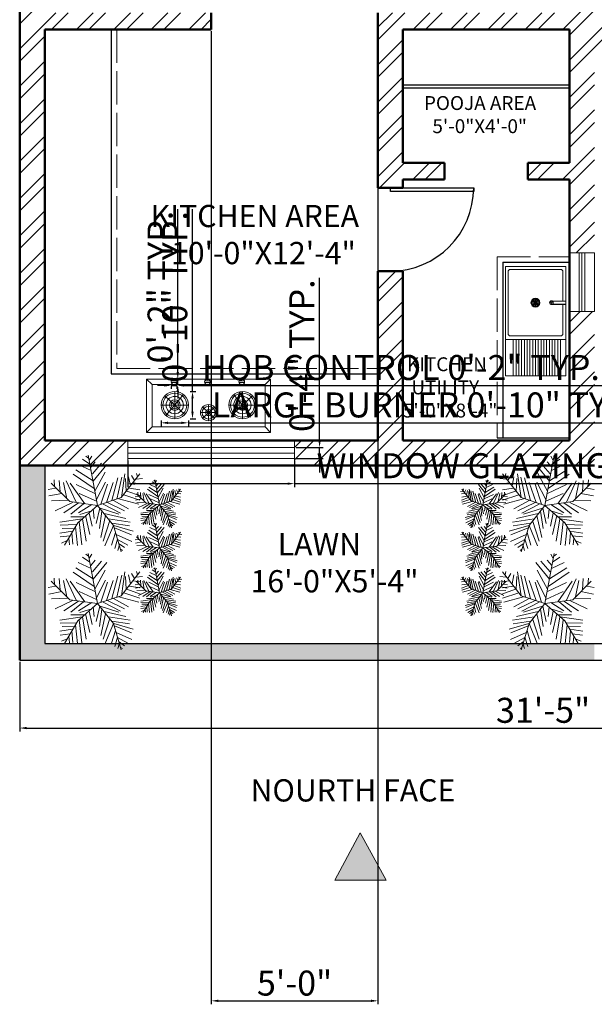
# Model space of a CAD drawing. Units: inches. Extents: x 764 to 1199, y 2696 to 3678.
# Tile 1 of 3: x 777 to 984, y 2696 to 3051. Entities that reach past the tile are written whole.
import ezdxf

# ---------------------------------------------------------------- set-up
doc = ezdxf.new("R2010")
doc.units = ezdxf.units.IN
doc.linetypes.add('ACAD_ISO02W100', pattern=[15, 12, -3])
for name, color, linetype, lineweight in [('A-ANNO-DIMS', 2, 'Continuous', 18), ('A-ANNO-SYMB', 7, 'Continuous', 18), ('A-ANNO-TEXT', 7, 'Continuous', 18), ('A-AREA-IDEN', 7, 'Continuous', 18), ('A-DOOR', 4, 'Continuous', 25), ('A-EQPM', 9, 'Continuous', 18), ('A-FIXT-PATT', 8, 'Continuous', 13), ('A-FLOR-FIXT', 8, 'Continuous', 20), ('A-GLAZ', 244, 'Continuous', 20), ('A-MILL', 8, 'Continuous', 25), ('A-MILL-HIDN', 8, 'ACAD_ISO02W100', 13), ('A-WALL', 7, 'Continuous', 50), ('A-WALL-PATT', 252, 'Continuous', 13), ('L-HRDS', 7, 'Continuous', 30), ('L-PLNT', 3, 'Continuous', 13)]:
    doc.layers.add(name, color=color, linetype=linetype, lineweight=lineweight)
doc.styles.get("Standard").update_dxf_attribs({"font": 'arial.ttf'})
doc.dimstyles.new('ISO-25', dxfattribs={"dimtxt": 9, "dimasz": 2.5, "dimexe": 1.25, "dimexo": 0.625, "dimtad": 1, "dimlunit": 3, "dimtxsty": 'Standard', "dimcen": 2.5, "dimadec": 0, "dimazin": 0, "dimtfac": 1, "dimtmove": 0, "dimatfit": 3, "dimfxl": 1, "dimarcsym": 0})

# ---------------------------------------------------------------- blocks, each defined once
blk = doc.blocks.new('*U5')
for p, q in [((-40, -1.47e-14), (-40, 5.999999999999984)), ((0, 0), (0, 5.999999999999999))]:
    blk.add_line(p, q)
blk.add_lwpolyline([(0, 0), (7.1e-15, -40), (-1.749999999999992, -40), (-1.75, -1e-16)], close=True)
blk.add_arc((0, 0), 40, 180, 270)
blk = doc.blocks.new('*U13')
for p, q in [((-10.18600000000015, 53.63999999999987), (-13.08399999999983, 55.96199999999976)), ((0, 0), (-10.5, 57)), ((-9.098999999999705, 51.7819999999997), (-6.563000000000101, 55.96199999999976)), ((-7.28800000000001, 39.70699999999965), (-21.77800000000025, 46.67299999999977)), ((-8.736999999999625, 47.13799999999969), (-17.06899999999996, 52.71100000000001)), ((-7.65000000000009, 43.42299999999977), (-2.577999999999974, 49.45999999999981)), ((-5.838999999999941, 35.99199999999973), (4.666999999999916, 48.06699999999977)), ((-5.114000000000032, 27.63199999999983), (10.46300000000019, 46.67299999999977)), ((-3.665000000000418, 19.27299999999968), (-27.57400000000007, 35.52699999999982)), ((-5.114000000000032, 28.09699999999975), (-24.67599999999993, 40.63599999999996)), ((-2.940999999999803, 16.48599999999987), (8.652000000000044, 37.84999999999991)), ((27, 9), (48, 36)), ((27.12699999999995, 9.05600000000004), (31.11200000000008, 35.99199999999973)), ((38.71900000000005, 34.13399999999979), (41.97899999999981, 28.56099999999992)), ((44.15300000000025, 36.45599999999991), (45.23900000000003, 32.74099999999999)), ((-31.5, 4.5), (-52.5, 25.5)), ((-48.58500000000003, 21.13099999999986), (-49.30899999999974, 29.02600000000007)), ((-43.51299999999992, 28.56099999999992), (-42.42699999999968, 15.55799999999976)), ((-38.44199999999955, 26.23899999999981), (-34.81899999999996, 7.662999999999783)), ((-35.54399999999987, 28.09699999999975), (-24.31399999999985, 3.946999999999661)), ((-14.5329999999999, 2.089999999999918), (-30.83399999999983, 25.30999999999995)), ((-24.31399999999985, 23.91699999999969), (-2.940999999999803, 13.69999999999982)), ((-1.128999999999905, 6.733999999999923), (9.014000000000124, 26.70399999999995)), ((3.942000000000007, 1.625), (11.1869999999999, 24.38099999999986)), ((10.10100000000011, 3.482999999999719), (17.70800000000008, 26.23899999999981)), ((16.25900000000001, 5.804999999999836), (23.14199999999983, 31.34799999999973)), ((22.05499999999984, 7.197999999999865), (27.48900000000003, 32.27699999999982)), ((31.83600000000024, 30.88299999999981), (32.56100000000015, 16.48599999999987)), ((35.09600000000001, 32.74099999999999), (37.26999999999998, 22.52399999999989)), ((40.52999999999975, 25.77499999999986), (48.86200000000008, 24.846)), ((43.79100000000017, 29.95399999999995), (51.03600000000006, 30.88299999999981)), ((-47.49800000000004, 19.73699999999962), (-55.83000000000038, 18.34399999999982)), ((-40.61500000000023, 13.69999999999982), (-55.10500000000002, 10.91299999999978)), ((-20.69099999999981, 13.69999999999982), (-1.128999999999905, 4.875999999999976)), ((29.66199999999981, 12.30699999999979), (48.13699999999972, 6.268999999999778)), ((33.28499999999986, 16.48599999999987), (48.86200000000008, 10.91299999999978)), ((36.18300000000045, 19.73699999999962), (48.13699999999972, 17.87999999999988)), ((-33.37000000000035, 6.268999999999778), (-52.20699999999988, 5.339999999999918)), ((-28.29899999999998, 3.482999999999719), (-47.86000000000012, -5.805000000000063)), ((-21.41600000000017, 3.017999999999801), (-38.07899999999973, -8.128000000000384)), ((0, 0), (-31.5, 4.5)), ((-15.98199999999951, 2.089999999999918), (-30.11000000000013, -9.521000000000186)), ((0, 0), (-22.5, -19.5)), ((-6.563000000000101, 1.161000000000058), (-21.41600000000017, -8.128000000000384)), ((0, 0), (27, 9)), ((0, 0), (18, -22.5)), ((6.478000000000065, 1.625), (26.03999999999996, -8.592000000000326)), ((11.1869999999999, 3.482999999999719), (30.74900000000025, -5.805000000000063)), ((18.06999999999971, 5.804999999999836), (35.09600000000001, -3.483000000000174)), ((24.22899999999982, 7.662999999999783), (46.6880000000001, 1.625)), ((-6.563000000000101, -5.805000000000063), (-19.96699999999964, -9.985000000000127)), ((-9.460999999999785, -8.592000000000326), (-6.201000000000021, -23.4530000000002)), ((-4.751999999999952, -3.483000000000174), (-3.665000000000418, -14.62900000000013)), ((2.493000000000392, -3.019000000000005), (-1.490999999999985, -20.20200000000023)), ((1.769000000000232, -2.555000000000063), (24.22899999999982, -9.521000000000186)), ((5.028999999999996, -6.270000000000209), (2.131000000000312, -25.77500000000009)), ((7.564999999999599, -9.056000000000267), (32.19800000000032, -14.62900000000013)), ((-17.43100000000004, -15.09400000000005), (-42.78899999999976, -18.80899999999997)), ((-24.31399999999985, -21.59600000000023), (-42.42699999999968, -22.06000000000017)), ((-22.5, -19.5), (-37.5, -45)), ((-15.2569999999996, -12.77200000000016), (-30.11000000000013, -12.77200000000016)), ((-20.69099999999981, -18.34500000000003), (-17.79300000000012, -44.35200000000032)), ((-17.06899999999996, -15.09400000000005), (-12.721, -40.17200000000025)), ((-13.44599999999991, -11.37800000000038), (-8.736999999999625, -32.74100000000021)), ((9.014000000000124, -11.37800000000038), (3.579999999999927, -35.99200000000019)), ((14.08499999999958, -16.95100000000025), (6.478000000000065, -40.17200000000025)), ((12.27399999999988, -15.09400000000005), (36.9069999999997, -18.80899999999997)), ((16.25900000000001, -19.73800000000028), (36.18300000000045, -22.98900000000003)), ((-28.29899999999998, -29.02600000000007), (-42.78899999999976, -31.34800000000018)), ((-26.8489999999997, -26.24000000000001), (-40.25300000000015, -25.77500000000009)), ((-29.02300000000014, -30.88400000000002), (-27.93600000000015, -43.88700000000016)), ((-25.03800000000001, -23.91800000000035), (-22.86500000000024, -45.28100000000017)), ((18.06999999999971, -22.52400000000012), (8.289000000000215, -45.74500000000012)), ((20.24400000000014, -30.4190000000001), (15.89699999999993, -44.81600000000026)), ((18, -22.5), (27, -52.5)), ((18.43300000000045, -22.52400000000012), (40.52999999999975, -29.02600000000007)), ((19.1569999999997, -25.31100000000015), (38.71900000000005, -33.20600000000013)), ((21.33100000000013, -32.74100000000021), (39.08100000000013, -40.63600000000019)), ((-30.83399999999983, -34.13499999999999), (-42.42699999999968, -35.52800000000025)), ((-34.45699999999988, -39.70800000000031), (-40.97800000000006, -42.49400000000014)), ((-32.64600000000019, -36.92100000000005), (-31.92099999999982, -44.35200000000032)), ((22.77999999999975, -37.85000000000014), (19.51900000000023, -48.53200000000015)), ((22.77999999999975, -38.31400000000008), (34.37199999999985, -44.81600000000026)), ((24.59100000000035, -43.42300000000022), (30.74900000000025, -47.60300000000029)), ((24.59100000000035, -45.74500000000012), (23.14199999999983, -50.85400000000004)), ((26.76400000000012, -49.92500000000018), (28.21300000000019, -50.85400000000004))]:
    blk.add_line(p, q)
blk = doc.blocks.new('*D14')
at = {"layer": 'A-ANNO-DIMS', "color": 0, "lineweight": -2, "transparency": 16777216}
for p, q in [((777.2372615392014, 2819.625478579777), (777.2372615392014, 2794.515568669596)), ((1154.237261539201, 2819.625478579777), (1154.237261539201, 2794.515568669596)), ((779.7372615392014, 2795.765568669596), (1151.737261539201, 2795.765568669596))]:
    blk.add_line(p, q, dxfattribs=at)
at = {"layer": 'A-ANNO-DIMS', "color": 0, "transparency": 16777216}
for points in [[(779.7372615392014, 2796.182235336263), (779.7372615392014, 2795.34890200293), (777.2372615392014, 2795.765568669596)], [(1151.737261539201, 2796.182235336263), (1151.737261539201, 2795.34890200293), (1154.237261539201, 2795.765568669596)]]:
    blk.add_solid(points, dxfattribs=at)
at = {"layer": 'Defpoints', "color": 0, "transparency": 16777216}
for p in [(777.2372615392014, 2820.250478579778), (1154.237261539201, 2820.250478579778), (1154.237261539201, 2795.765568669596)]:
    blk.add_point(p, dxfattribs=at)
at = {"layer": 'A-ANNO-DIMS', "color": 0, "transparency": 16777216, "insert": (965.7372615392015, 2800.988795136172), "char_height": 9, "attachment_point": 5}
blk.add_mtext('31\'-5"', dxfattribs=at)
blk = doc.blocks.new('WIN-GLAZING-60IN')
for p, q in [((0.0002615392013468, 4.000478579777791), (60.00026153920135, 4.000478579777791)), ((0.0002615392013468, 2.000478579777791), (60.00026153920135, 2.000478579777791)), ((0.0002615392013468, 0.0004785797777913), (60.00026153920135, 0.0004785797777913))]:
    blk.add_line(p, q)
blk = doc.blocks.new('VENT-GLAZING-21IN')
for p, q in [((0.0002615392015741, 0.0004785797773366), (0.0002615392015741, 21.00047857977734)), ((1.000261539201574, 0.0004785797773366), (1.000261539201574, 21.00047857977734)), ((2.000261539201574, 0.0004785797773366), (2.000261539201574, 21.00047857977734))]:
    blk.add_line(p, q)
blk = doc.blocks.new('COOKTOP-BURNER-LARGE')
for p, q in [((8.519274616664575, 1.570641359189266), (1.313840023247735, 8.261224759886773)), ((1.758228681000105, 1.148240305507442), (8.074885958912205, 8.683625813568597)), ((4.916557319956154, 9.832288262371094), (4.916557319956154, -0.0004221432950544)), ((0.0002021171230808, 4.915933059538019), (9.83291252278923, 4.915933059538019))]:
    blk.add_line(p, q)
for radius in [4.916355202833074, 4.316355202833074, 3.116355202833074, 1.916355202833074, 1.316355202833074]:
    blk.add_circle((4.916557319956154, 4.915933059538019), radius)
blk = doc.blocks.new('COOKTOP-CONTROL')
for p, q in [((0.0453271065459831, 1.317444336811149), (1.989388325886238, 1.317444336811604)), ((0.0453271065460967, 0.7174443368112406), (1.989388325886238, 0.7174443368112406))]:
    blk.add_line(p, q)
blk.add_circle((1.01735771621611, 1.017444336811422), 1.017272582022997)
for start, end in [(45.96822923670138, 134.0317707633033), (225.9682292368025, 314.0317707631974)]:
    blk.add_arc((1.01735771621611, 1.017444336811422), 0.4172725820229971, start, end)
blk = doc.blocks.new('*D24')
at = {"layer": 'A-ANNO-DIMS', "color": 0, "lineweight": -2, "transparency": 16777216}
for p, q in [((816.2372615392019, 2892.125478579778), (816.2372615392019, 2882.500478579778)), ((876.237261539202, 2892.125478579778), (876.237261539202, 2882.500478579778)), ((818.7372615392019, 2883.750478579778), (873.737261539202, 2883.750478579778)), ((876.237261539202, 2883.750478579778), (1052.558885004413, 2883.750478579778))]:
    blk.add_line(p, q, dxfattribs=at)
at = {"layer": 'A-ANNO-DIMS', "color": 0, "transparency": 16777216}
for points in [[(818.7372615392019, 2884.167145246444), (818.7372615392019, 2883.333811913111), (816.2372615392019, 2883.750478579778)], [(873.737261539202, 2884.167145246444), (873.737261539202, 2883.333811913111), (876.237261539202, 2883.750478579778)]]:
    blk.add_solid(points, dxfattribs=at)
at = {"layer": 'Defpoints', "color": 0, "transparency": 16777216}
for p in [(816.2372615392019, 2892.750478579778), (876.237261539202, 2892.750478579778), (876.237261539202, 2883.750478579778)]:
    blk.add_point(p, dxfattribs=at)
at = {"layer": 'A-ANNO-DIMS', "color": 0, "transparency": 16777216, "insert": (965.6480732718076, 2889.032027010883), "char_height": 9, "attachment_point": 5}
blk.add_mtext('WINDOW GLAZING 5\'-0" TYP.', dxfattribs=at)
blk = doc.blocks.new('*D25')
at = {"layer": 'A-ANNO-DIMS', "color": 0, "lineweight": -2, "transparency": 16777216}
for p, q in [((885.2372615392029, 2899.250478579779), (885.2372615392029, 2957.859960162317)), ((876.8622615392024, 2896.750478579779), (886.4872615392028, 2896.750478579779)), ((885.2372615392029, 2892.750478579779), (885.2372615392029, 2896.750478579779)), ((876.8622615392024, 2892.750478579779), (886.4872615392028, 2892.750478579779)), ((885.2372615392029, 2890.250478579779), (885.2372615392029, 2887.750478579779))]:
    blk.add_line(p, q, dxfattribs=at)
at = {"layer": 'A-ANNO-DIMS', "color": 0, "transparency": 16777216}
for points in [[(884.8205948725363, 2899.250478579779), (885.6539282058696, 2899.250478579779), (885.2372615392029, 2896.750478579779)], [(884.8205948725363, 2890.250478579779), (885.6539282058696, 2890.250478579779), (885.2372615392029, 2892.750478579779)]]:
    blk.add_solid(points, dxfattribs=at)
at = {"layer": 'Defpoints', "color": 0, "transparency": 16777216}
for p in [(876.2372615392024, 2896.750478579779), (885.2372615392029, 2896.750478579779), (876.2372615392024, 2892.750478579779)]:
    blk.add_point(p, dxfattribs=at)
at = {"layer": 'A-ANNO-DIMS', "color": 0, "transparency": 16777216, "insert": (880.0171046497084, 2929.805219371047), "char_height": 9, "attachment_point": 5, "rotation": 90}
blk.add_mtext('0\'-4" TYP.', dxfattribs=at)
blk = doc.blocks.new('*D28')
at = {"layer": 'A-ANNO-DIMS', "color": 0, "lineweight": -2, "transparency": 16777216}
for p, q in [((829.3360851341931, 2919.092989980183), (826.8360851341931, 2919.092989980183)), ((831.8360851341932, 2919.092989980183), (833.8706302982391, 2919.092989980183)), ((831.8360851341932, 2918.77317175479), (831.8360851341932, 2917.842989980183)), ((833.8706302982391, 2918.77317175479), (833.8706302982391, 2917.842989980183)), ((836.3706302982391, 2919.092989980183), (990.1983929176115, 2919.092989980183))]:
    blk.add_line(p, q, dxfattribs=at)
at = {"layer": 'A-ANNO-DIMS', "color": 0, "transparency": 16777216}
for points in [[(829.3360851341931, 2919.50965664685), (829.3360851341931, 2918.676323313516), (831.8360851341932, 2919.092989980183)], [(836.3706302982391, 2919.50965664685), (836.3706302982391, 2918.676323313516), (833.8706302982391, 2919.092989980183)]]:
    blk.add_solid(points, dxfattribs=at)
at = {"layer": 'Defpoints', "color": 0, "transparency": 16777216}
for p in [(831.8360851341932, 2919.39817175479), (833.8706302982391, 2919.39817175479), (833.8706302982391, 2919.092989980183)]:
    blk.add_point(p, dxfattribs=at)
at = {"layer": 'A-ANNO-DIMS', "color": 0, "transparency": 16777216, "insert": (914.5345116079253, 2924.374538411288), "char_height": 9, "attachment_point": 5}
blk.add_mtext('HOB CONTROL 0\'-2" TYP.', dxfattribs=at)
blk = doc.blocks.new('*D29')
at = {"layer": 'A-ANNO-DIMS', "color": 0, "lineweight": -2, "transparency": 16777216}
for p, q in [((834.175812072847, 2923.932716918836), (834.175812072847, 2982.542198501374)), ((834.175812072847, 2919.39817175479), (834.175812072847, 2921.432716918836)), ((834.4956302982396, 2921.432716918836), (835.425812072847, 2921.432716918836)), ((834.175812072847, 2916.898171754791), (834.175812072847, 2914.398171754791)), ((834.4956302982396, 2919.39817175479), (835.425812072847, 2919.39817175479))]:
    blk.add_line(p, q, dxfattribs=at)
at = {"layer": 'A-ANNO-DIMS', "color": 0, "transparency": 16777216}
for points in [[(833.7591454061803, 2923.932716918836), (834.5924787395135, 2923.932716918836), (834.175812072847, 2921.432716918836)], [(833.7591454061803, 2916.898171754791), (834.5924787395135, 2916.898171754791), (834.175812072847, 2919.39817175479)]]:
    blk.add_solid(points, dxfattribs=at)
at = {"layer": 'Defpoints', "color": 0, "transparency": 16777216}
for p in [(833.8706302982396, 2921.432716918836), (834.175812072847, 2921.432716918836), (833.8706302982396, 2919.39817175479)]:
    blk.add_point(p, dxfattribs=at)
at = {"layer": 'A-ANNO-DIMS', "color": 0, "transparency": 16777216, "insert": (828.9556551833523, 2954.487457710105), "char_height": 9, "attachment_point": 5, "rotation": 90}
blk.add_mtext('0\'-2" TYP.', dxfattribs=at)
blk = doc.blocks.new('*D32')
at = {"layer": 'A-ANNO-DIMS', "color": 0, "lineweight": -2, "transparency": 16777216}
for p, q in [((828.174202117123, 2906.483577856705), (828.174202117123, 2904.383671295855)), ((838.006912522789, 2906.483577856705), (838.006912522789, 2904.383671295855)), ((830.674202117123, 2905.633671295855), (835.506912522789, 2905.633671295855)), ((838.006912522789, 2905.633671295855), (1005.911755633294, 2905.633671295855))]:
    blk.add_line(p, q, dxfattribs=at)
at = {"layer": 'A-ANNO-DIMS', "color": 0, "transparency": 16777216}
for points in [[(830.674202117123, 2906.050337962522), (830.674202117123, 2905.217004629188), (828.174202117123, 2905.633671295855)], [(835.506912522789, 2906.050337962522), (835.506912522789, 2905.217004629188), (838.006912522789, 2905.633671295855)]]:
    blk.add_solid(points, dxfattribs=at)
at = {"layer": 'Defpoints', "color": 0, "transparency": 16777216}
for p in [(828.174202117123, 2907.108577856705), (838.006912522789, 2907.108577856705), (838.006912522789, 2905.633671295855)]:
    blk.add_point(p, dxfattribs=at)
at = {"layer": 'A-ANNO-DIMS', "color": 0, "transparency": 16777216, "insert": (923.2093340780414, 2910.91215014988), "char_height": 9, "attachment_point": 5}
blk.add_mtext('LARGE BURNER 0\'-10" TYP.', dxfattribs=at)
blk = doc.blocks.new('*D33')
at = {"layer": 'A-ANNO-DIMS', "color": 0, "lineweight": -2, "transparency": 16777216}
for p, q in [((839.48181908364, 2916.941288262372), (839.48181908364, 2982.543266434269)), ((838.6319125227895, 2916.941288262372), (840.73181908364, 2916.941288262372)), ((839.48181908364, 2909.608577856706), (839.48181908364, 2914.441288262372)), ((838.6319125227895, 2907.108577856706), (840.73181908364, 2907.108577856706))]:
    blk.add_line(p, q, dxfattribs=at)
at = {"layer": 'A-ANNO-DIMS', "color": 0, "transparency": 16777216}
for points in [[(839.0651524169733, 2914.441288262372), (839.8984857503066, 2914.441288262372), (839.48181908364, 2916.941288262372)], [(839.0651524169733, 2909.608577856706), (839.8984857503066, 2909.608577856706), (839.48181908364, 2907.108577856706)]]:
    blk.add_solid(points, dxfattribs=at)
at = {"layer": 'Defpoints', "color": 0, "transparency": 16777216}
for p in [(838.0069125227895, 2916.941288262372), (839.48181908364, 2916.941288262372), (838.0069125227895, 2907.108577856706)]:
    blk.add_point(p, dxfattribs=at)
at = {"layer": 'A-ANNO-DIMS', "color": 0, "transparency": 16777216, "insert": (834.2616621941454, 2950.99227734832), "char_height": 9, "attachment_point": 5, "rotation": 90}
blk.add_mtext('0\'-10" TYP.', dxfattribs=at)
blk = doc.blocks.new('*D36')
at = {"layer": 'A-ANNO-DIMS', "color": 0, "lineweight": -2, "transparency": 16777216}
for p, q in [((846.237262, 3046.625479), (846.237262, 2696.328067)), ((906.2372619999999, 3046.625479), (906.2372619999999, 2696.328067)), ((848.737262, 2697.578067), (903.7372619999999, 2697.578067))]:
    blk.add_line(p, q, dxfattribs=at)
at = {"layer": 'A-ANNO-DIMS', "color": 0, "transparency": 16777216}
for points in [[(848.737262, 2697.994733666666), (848.737262, 2697.161400333334), (846.237262, 2697.578067)], [(903.7372619999999, 2697.994733666666), (903.7372619999999, 2697.161400333334), (906.2372619999999, 2697.578067)]]:
    blk.add_solid(points, dxfattribs=at)
at = {"layer": 'Defpoints', "color": 0, "transparency": 16777216}
for p in [(846.237262, 3047.250479), (906.2372619999999, 3047.250479), (906.2372619999999, 2697.578067)]:
    blk.add_point(p, dxfattribs=at)
at = {"layer": 'A-ANNO-DIMS', "color": 0, "transparency": 16777216, "insert": (876.237262, 2702.798223889495), "char_height": 9, "attachment_point": 5}
blk.add_mtext('5\'-0"', dxfattribs=at)

msp = doc.modelspace()

# ---------------------------------------------------------------- hatches: boundary and pattern name
at = {"layer": 'A-ANNO-SYMB'}
h = msp.add_hatch(color=256, dxfattribs=at)
h.dxf.hatch_style = 1
h.paths.add_polyline_path([(899.8408897103933, 2758.076893952801), (890.7054604401357, 2740.978067102982), (909.2115573473543, 2740.978067102982)])
h.paths.add_polyline_path([(1023.879118762197, 3009.352008593085), (1018.595038768721, 3000.199713573126), (1029.163198755673, 3000.199713573126)])
h.paths.add_polyline_path([(856.904311954004, 3232.137894596994), (851.9031607095966, 3229.250478579777), (856.9043119540038, 3226.363062562561)])
at = {"layer": 'A-FIXT-PATT'}
h = msp.add_hatch(dxfattribs=at)
h.set_pattern_fill('ANSI31', color=256, scale=0.3149606299212598, angle=45, style=0)
h.set_pattern_definition([(90, (0, 0), (-1, 0), [])])
h.paths.add_polyline_path([(954.0537529999999, 2922.503875), (972.0537529999999, 2922.503875), (972.0537529999999, 2935.684321), (954.0537529999999, 2935.684321)])
at = {"layer": 'A-WALL-PATT'}
h = msp.add_hatch(dxfattribs=at)
h.set_pattern_fill('ANSI32', color=256)
h.set_pattern_definition([(45, (0, 0), (-6.735192090801866, 6.735192090801866), []), (45, (4.49013, 0), (-6.735192090801866, 6.735192090801866), [])])
h.paths.add_polyline_path([(975.2372615392017, 2999.250478579778), (960.2372615392013, 2999.250478579778), (960.2372615392013, 2993.250478579778), (975.2372615392017, 2993.250478579778), (975.2372615392015, 2966.770834040433), (984.2372615392013, 2966.770834040433), (984.2372615392013, 3039.250478579778), (987.2372615392013, 3039.250478579779), (987.2372615392013, 3043.750478579778), (987.2372615392013, 3048.250478579778), (984.2372615392013, 3048.250478579778), (984.2372615392013, 3053.250478579777), (984.2372615392013, 3077.250478579778), (975.2372615392014, 3077.250478579778), (975.2372615392014, 3053.250478579777), (915.2372615392017, 3053.250478579777), (906.2372615392017, 3053.250478579777), (906.2372615392017, 3047.250478579778), (906.2372615392017, 2990.250478579778), (910.7372615392017, 2990.250478579778), (915.2372615392017, 2990.250478579778), (915.2372615392017, 2993.250478579778), (930.2372615392014, 2993.250478579778), (930.2372615392014, 2999.250478579778), (915.2372615392017, 2999.250478579778), (915.2372615392017, 3047.250478579778), (975.237261539201, 3047.250478579778)])
h.paths.add_polyline_path([(1047.237261539201, 3048.250478579778), (1047.237261539201, 3043.750478579778), (1047.237261539201, 3039.250478579779), (1066.237261539201, 3039.250478579778), (1066.237261539201, 3048.250478579778)])
h.paths.add_polyline_path([(906.2372615392014, 2899.250478579777), (876.2372615392013, 2899.250478579777), (876.2372615392013, 2890.250478579778), (984.2372615392013, 2890.250478579778), (984.2372615392013, 2945.770834040434), (975.2372615392015, 2945.770834040434), (975.2372615392014, 2899.250478579777), (915.2372615392014, 2899.250478579777), (915.2372615392017, 2960.250478579777), (906.2372615392012, 2960.250478579777)])
h.paths.add_polyline_path([(786.2372615392021, 3047.250478579778), (846.2372615392014, 3047.250478579778), (846.2372615392014, 3053.250478579777), (786.2372615392015, 3053.250478579777), (786.2372615392015, 3247.250478579778), (915.2372615392019, 3247.250478579778), (915.2372615392019, 3259.250478579777), (906.2372615392019, 3259.250478579777), (906.2372615392019, 3256.250478579777), (839.2372615392017, 3256.250478579777), (839.2372615392017, 3271.750478579777), (830.2372615392014, 3271.750478579777), (830.2372615392014, 3256.250478579777), (786.2372615392015, 3256.250478579777), (786.2372615392015, 3308.250478579778), (830.2372615392014, 3308.250478579778), (830.2372615392014, 3292.750478579777), (839.2372615392017, 3292.750478579777), (839.2372615392017, 3308.250478579778), (906.2372615392018, 3308.250478579777), (906.2372615392018, 3289.250478579778), (915.2372615392019, 3289.250478579778), (915.2372615392017, 3320.250478579777), (906.2372615392018, 3320.250478579777), (906.2372615392018, 3317.250478579778), (786.2372615392015, 3317.250478579778), (786.2372615392015, 3336.750478579778), (777.2372615392014, 3336.750478579778), (777.2372615392014, 2890.250478579778), (816.2372615392014, 2890.250478579778), (816.2372615392014, 2899.250478579777), (786.2372615392014, 2899.250478579777)])
h.paths.add_polyline_path([(979.2372615392013, 3443.250478579778), (997.7372615392013, 3443.250478579778), (997.7372615392013, 3452.250478579777), (979.2372615392014, 3452.250478579777), (979.2372615392014, 3455.250478579777), (970.2372615392011, 3455.250478579777), (970.2372615392011, 3386.250478579778), (967.2372615392012, 3386.250478579778), (967.2372615392012, 3377.250478579777), (970.2372615392011, 3377.250478579777), (970.2372615392011, 3290.250478579777), (979.2372615392013, 3290.250478579777)])
h.paths.add_polyline_path([(777.2372615392014, 3357.750478579777), (786.2372615392014, 3357.750478579777), (786.2372615392014, 3377.250478579777), (906.2372615392014, 3377.250478579777), (906.2372615392017, 3350.250478579777), (915.2372615392017, 3350.250478579777), (915.2372615392014, 3377.250478579777), (931.2372615392012, 3377.250478579777), (931.2372615392012, 3386.250478579778), (786.2372615392014, 3386.250478579778), (786.2372615392014, 3542.250478579778), (970.2372615392015, 3542.250478579778), (970.2372615392015, 3485.250478579778), (979.2372615392014, 3485.250478579778), (979.2372615392014, 3542.250478579778), (979.2372615392014, 3551.250478579778), (777.2372615392014, 3551.250478579778)])
h.paths.add_polyline_path([(1076.237261539201, 3452.250478579778), (1057.737261539201, 3452.250478579778), (1057.737261539201, 3443.250478579777), (1076.237261539201, 3443.250478579777), (1088.237261539201, 3443.250478579777), (1088.237261539201, 3452.250478579777), (1085.237261539201, 3452.250478579777), (1085.237261539201, 3517.522907527973), (1076.237261539201, 3517.522907527973)])
h.paths.add_polyline_path([(913.697357037155, 2904.723445549297), (949.0861701340172, 2904.723445549297), (949.0861701340172, 2931.714123130015), (913.697357037155, 2931.714123130015)], flags=24)
h = msp.add_hatch(color=256, dxfattribs=at)
h.dxf.hatch_style = 1
h.paths.add_polyline_path([(1076.237261539201, 3551.250478579778), (979.2372615392014, 3551.250478579778), (979.2372615392014, 3542.250478579778), (1076.237261539201, 3542.250478579778)])
h.paths.add_polyline_path([(786.2372615392014, 2826.250478579777), (786.2372615392015, 2890.250478579778), (777.2372615392014, 2890.250478579778), (777.2372615392014, 2820.250478579778), (984.2372615392013, 2820.250478579778), (984.2372615392013, 2826.250478579778)])
h.paths.add_polyline_path([(1154.237261539201, 3039.250478579778), (1145.237261539201, 3039.250478579778), (1145.237261539201, 2826.250478579779), (1136.237261539201, 2826.250478579779), (1136.237261539201, 2820.250478579778), (1154.237261539201, 2820.250478579778)])

# ---------------------------------------------------------------- linework, layer by layer
at = {"layer": 'A-ANNO-SYMB'}
msp.add_lwpolyline([(899.8408897103933, 2758.076893952801), (890.7054604401357, 2740.978067102982), (909.2115573473543, 2740.978067102982)], close=True, dxfattribs=at)
at = {"layer": 'A-EQPM'}
for p, q in [((824.925282633565, 2919.398171754789), (822.9252826335651, 2921.398171754788)), ((865.6191033448049, 2919.398171754789), (867.6191033448048, 2921.398171754788)), ((847.3890313806887, 2907.292274934301), (843.1553545976813, 2911.313846214217)), ((843.1668584639428, 2907.280233294823), (847.3775275144271, 2911.325887853695)), ((845.2721929891849, 2912.222694740658), (845.2721929891849, 2906.38342640786)), ((842.3525588227857, 2909.303060574259), (848.1918271555841, 2909.303060574259)), ((824.925282633565, 2904.202320759576), (822.9252826335651, 2902.202320759576)), ((865.6191033448049, 2904.202320759576), (867.6191033448048, 2902.202320759576))]:
    msp.add_line(p, q, dxfattribs=at)
msp.add_lwpolyline([(833.1162081072982, 2921.398171754788), (867.6191033448048, 2921.398171754788), (867.6191033448048, 2902.202320759576), (822.9252826335651, 2902.202320759576), (822.9252826335651, 2921.398171754788), (832.5905073251341, 2921.398171754788)], dxfattribs=at)
msp.add_lwpolyline([(824.925282633565, 2919.398171754789), (865.6191033448049, 2919.398171754789), (865.6191033448049, 2904.202320759576), (824.925282633565, 2904.202320759576)], close=True, dxfattribs=at)
for radius in [2.919634166399191, 2.319634166399191, 1.119634166399191, 0.5196341663991914]:
    msp.add_circle((845.2721929891849, 2909.303060574259), radius, dxfattribs=at)
at = {"layer": 'A-FLOR-FIXT'}
for p, q in [((961.3842979439607, 2948.882607952027), (964.61481812946, 2948.882607952027)), ((964.4906556338229, 2948.261565986365), (961.5084604395978, 2949.503649917691)), ((961.5683797430296, 2948.133746243215), (964.430736330391, 2949.631469660841)), ((964.2141603290129, 2947.817804477784), (961.7849557444079, 2949.947411426272)), ((961.8843490923948, 2947.714115685153), (964.114766981026, 2950.051100218903)), ((963.667423061972, 2947.411886538822), (962.3316930114487, 2950.353329365233)), ((962.4630138622279, 2947.359064215846), (963.5361022111927, 2950.406151688209)), ((962.9995580367104, 2950.497868044778), (962.9995580367104, 2947.267347859278)), ((969.0559383443455, 2949.482607952028), (973.885470840207, 2949.482607952028)), ((969.1975238471161, 2949.382607952029), (973.885470840207, 2949.382607952028)), ((969.0559383443461, 2948.282607952028), (973.885470840207, 2948.282607952028)), ((969.1975238471169, 2948.382607952028), (973.885470840207, 2948.382607952028)), ((952.22203472822, 2935.684320602721), (973.885470840207, 2935.684320602721))]:
    msp.add_line(p, q, dxfattribs=at)
msp.add_lwpolyline([(952.22203472822, 2961.877842781751), (973.885470840207, 2961.877842781751), (973.885470840207, 2922.503874820434), (952.22203472822, 2922.503874820434)], close=True, dxfattribs=at)
msp.add_lwpolyline([(972.8617283619678, 2948.282607952028), (972.8617283619678, 2937.803836746899, -0.4142135623730951), (971.9617283619677, 2936.903836746898), (954.0373877114529, 2936.903836746898, -0.4142135623730951), (953.1373877114528, 2937.803836746899), (953.1373877114528, 2959.961379157157, -0.4142135623730581), (954.0373877114529, 2960.861379157157), (971.9617283619677, 2960.861379157157, -0.4142135623730951), (972.8617283619678, 2959.961379157157), (972.8617283619678, 2949.482607952028)], format="xyb", dxfattribs=at)
for centre, radius in [((962.9995580367104, 2948.882607952027), 1.615260092749667), ((962.9995580367104, 2948.882607952027), 1.315260092749667), ((968.7382732457139, 2948.882607952027), 0.6789043488511198), ((968.7382732457139, 2948.882607952027), 0.2789043488511197)]:
    msp.add_circle(centre, radius, dxfattribs=at)
at = {"layer": 'A-GLAZ'}
for points in [[(984.2372615392013, 2966.770834040433), (984.2372615392013, 2945.770834040434), (975.2372615392014, 2945.770834040434), (975.2372615392014, 2966.770834040433)], [(816.2372615392014, 2899.250478579777), (876.2372615392013, 2899.250478579777), (876.2372615392013, 2890.250478579778), (816.2372615392014, 2890.250478579778)]]:
    msp.add_lwpolyline(points, close=True, dxfattribs=at)
at = {"layer": 'A-MILL'}
for p, q in [((810.2372615392015, 3047.250478579778), (810.2372615392013, 2923.250478579777)), ((915.2372615392017, 3027.250478579778), (975.2372615392014, 3027.250478579778)), ((915.2372615392017, 3026.250478579778), (975.2372615392014, 3026.250478579778)), ((951.2372615392015, 2963.432429559658), (951.2372615392015, 2900.250478579778)), ((951.2372615392017, 2963.432429559658), (975.2372615392017, 2963.432429559658)), ((810.2372615392013, 2923.250478579777), (906.2372615392017, 2923.250478579777)), ((949.2372615392014, 2900.250478579778), (975.2372615392014, 2900.250478579778))]:
    msp.add_line(p, q, dxfattribs=at)
at = {"layer": 'A-MILL-HIDN'}
for p, q in [((812.2372615392015, 3047.250478579778), (812.2372615392013, 2925.250478579777)), ((949.2372615392017, 2965.432429559658), (949.2372615392014, 2900.250478579778)), ((949.2372615392017, 2965.432429559658), (975.2372615392017, 2965.432429559658)), ((812.2372615392011, 2925.250478579777), (906.2372615392017, 2925.250478579778))]:
    msp.add_line(p, q, dxfattribs=at)
at = {"layer": 'A-WALL'}
for p, q in [((777.2372615392014, 3551.250478579778), (777.2372615392014, 2820.250478579778)), ((846.2372615392014, 3047.250478579778), (846.2372615392014, 3053.250478579777)), ((906.2372615392017, 3047.250478579778), (906.2372615392017, 3053.250478579777)), ((786.2372615392014, 3047.250478579778), (846.2372615392014, 3047.250478579778)), ((786.2372615392015, 3047.250478579778), (786.2372615392014, 2899.250478579777)), ((906.2372615392017, 3047.250478579778), (906.2372615392017, 2990.250478579778)), ((915.2372615392017, 3047.250478579777), (915.2372615392017, 2999.250478579778)), ((915.2372615392017, 3047.250478579778), (975.2372615392014, 3047.250478579778)), ((975.237261539201, 3047.250478579778), (975.2372615392017, 2999.250478579778)), ((915.2372615392017, 2999.250478579778), (930.2372615392014, 2999.250478579778)), ((930.2372615392014, 2993.250478579778), (930.2372615392014, 2999.250478579778)), ((960.2372615392013, 2993.250478579778), (960.2372615392013, 2999.250478579778)), ((960.2372615392013, 2999.250478579778), (975.2372615392014, 2999.250478579778)), ((915.2372615392017, 2993.250478579778), (930.2372615392014, 2993.250478579778)), ((915.2372615392017, 2993.250478579778), (915.2372615392017, 2990.250478579778)), ((960.2372615392013, 2993.250478579778), (975.2372615392014, 2993.250478579778)), ((975.2372615392017, 2993.250478579778), (975.2372615392014, 2899.250478579777)), ((915.2372615392017, 2990.250478579778), (906.2372615392017, 2990.250478579778)), ((906.2372615392012, 2960.250478579777), (906.2372615392014, 2899.250478579777)), ((915.2372615392017, 2960.250478579777), (906.2372615392017, 2960.250478579777)), ((915.2372615392017, 2960.250478579777), (915.2372615392014, 2899.250478579777)), ((786.2372615392014, 2899.250478579777), (906.2372615392017, 2899.250478579777)), ((915.2372615392017, 2899.250478579777), (975.2372615392014, 2899.250478579777)), ((777.2372615392014, 2890.250478579778), (984.2372615392013, 2890.250478579778))]:
    msp.add_line(p, q, dxfattribs=at)
at = {"layer": 'L-HRDS'}
for p, q in [((786.2372615392015, 2890.250478579778), (786.2372615392014, 2826.250478579777)), ((786.2372615392014, 2826.250478579777), (1145.237261539201, 2826.250478579779)), ((777.2372615392014, 2820.250478579778), (1154.237261539201, 2820.250478579778))]:
    msp.add_line(p, q, dxfattribs=at)

# ---------------------------------------------------------------- block references
at = {"layer": 'A-DOOR', "xscale": 0.7500000000000209, "yscale": 0.7500000000000209, "zscale": 0.7500000000000209, "rotation": 90}
msp.add_blockref('*U5', (910.7372615392017, 2990.250478579778), dxfattribs=at)
at = {"layer": 'A-EQPM'}
for name, p in [('COOKTOP-CONTROL', (831.836, 2919.398000000001)), ('COOKTOP-CONTROL', (843.8284471060148, 2919.398000000001)), ('COOKTOP-CONTROL', (856.1992713384576, 2919.398000000001)), ('COOKTOP-BURNER-LARGE', (828.1739999999999, 2907.109))]:
    msp.add_blockref(name, p, dxfattribs=at)
at = {"layer": 'A-EQPM', "extrusion": (0, 0, -1), "zscale": -1, "rotation": 180}
msp.add_blockref('COOKTOP-BURNER-LARGE', (-852.5372713384575, 2916.940866119077), dxfattribs=at)
at = {"layer": 'A-GLAZ'}
for name, p in [('VENT-GLAZING-21IN', (978.7369999999999, 2945.770355460656)), ('WIN-GLAZING-60IN', (816.2370000000006, 2892.75))]:
    msp.add_blockref(name, p, dxfattribs=at)
at = {"layer": 'L-PLNT'}
for p, xscale, yscale, zscale in [((805.2677837499818, 2875.842903767738), 0.3176375854075682, 0.3176375854075682, 0.3176375854075682), ((966.4045779064448, 2875.842903767738), -0.3176375854075682, 0.3176375854075682, 0.3176375854075682), ((827.5992516714927, 2876.102896613388), 0.1576419880843083, 0.1576419880843083, 0.1576419880843083), ((944.0731099849339, 2876.102896613389), -0.1576419880843083, 0.1576419880843083, 0.1576419880843083), ((827.5992516714925, 2860.581527235739), 0.1576419880843083, 0.1576419880843083, 0.1576419880843083), ((944.0731099849341, 2860.581527235739), -0.1576419880843083, 0.1576419880843083, 0.1576419880843083), ((805.2677837499818, 2840.544169923118), 0.3176375854075682, 0.3176375854075682, 0.3176375854075682), ((966.404577906445, 2840.544169923118), -0.3176375854075682, 0.3176375854075682, 0.3176375854075682), ((827.5992516714927, 2844.451785538212), 0.1576419880843083, 0.1576419880843083, 0.1576419880843083), ((944.0731099849339, 2844.451785538213), -0.1576419880843083, 0.1576419880843083, 0.1576419880843083)]:
    msp.add_blockref('*U13', p, dxfattribs=dict(at, xscale=xscale, yscale=yscale, zscale=zscale))

# ---------------------------------------------------------------- texts
at = {"layer": 'A-ANNO-TEXT', "insert": (860.3671560247709, 2777.332937943648), "char_height": 8, "attachment_point": 1}
msp.add_mtext_dynamic_manual_height_columns('NOURTH FACE', width=82.862988265495, gutter_width=12.5, heights=[0], dxfattribs=at)
at = {"layer": 'A-AREA-IDEN', "attachment_point": 1}
for s, width, insert, char_height in [('POOJA AREA\\P  5\'-0"X4\'-0"', 44.79937515122037, (922.8221032432756, 3023.250478579778), 5), ('KITCHEN AREA\\P   10\'-0"X12\'-4"', 83.57450490122028, (824.3894447467447, 2984.076052913271), 8), (' KITCHEN \\P  UTILITY\\P5\'-0"X8\'-4"', 33.58956758307795, (915.2372615392014, 2929.226060374217), 5), ('    LAWN\\P16\'-0"X5\'-4"', 56.27908817528259, (860.3671560247709, 2865.94901319582), 8)]:
    msp.add_mtext_dynamic_manual_height_columns(s, width=width, gutter_width=12.5, heights=[0], dxfattribs=dict(at, insert=insert, char_height=char_height))

# ---------------------------------------------------------------- dimensions: what is measured, and where the dimension line sits
at = {"layer": 'A-ANNO-DIMS'}
for base, p1, p2, override, picture, middle in [((906.2372619999999, 2697.578067), (846.237262, 3047.250479), (906.2372619999999, 3047.250479), {"dimdec": 1, "dimlfac": 1, "dimrnd": 0, "dimzin": 1, "dimdsep": 46, "dimlunit": 4, "dimfrac": 2}, '*D36', (876.237262, 2702.798223889495)), ((1154.237261539201, 2795.765568669596), (777.2372615392014, 2820.250478579778), (1154.237261539201, 2820.250478579778), {"dimclrd": 0, "dimclre": 0, "dimclrt": 0}, '*D14', (965.7372615392015, 2800.988795136172))]:
    dim = msp.add_linear_dim(base=base, p1=p1, p2=p2, dimstyle='ISO-25', override=override, dxfattribs=at)
    dim.commit()
    dim.dimension.update_dxf_attribs({"geometry": picture, "text_midpoint": middle})
for base, p1, p2, picture, middle in [((834.175812072847, 2921.432716918836), (833.8706302982391, 2919.39817175479), (833.8706302982391, 2921.432716918836), '*D29', (828.9556551833523, 2954.487457710105)), ((839.48181908364, 2916.941288262372), (838.006912522789, 2907.108577856705), (838.006912522789, 2916.941288262371), '*D33', (834.2616621941454, 2950.99227734832)), ((885.2372615392029, 2896.750478579779), (876.237261539202, 2892.750478579778), (876.237261539202, 2896.750478579778), '*D25', (880.0171046497084, 2929.805219371047))]:
    dim = msp.add_linear_dim(base=base, p1=p1, p2=p2, angle=90, text='<> TYP.', dimstyle='ISO-25', override={"dimdec": 1, "dimlfac": 1, "dimrnd": 0, "dimzin": 1, "dimdsep": 46, "dimlunit": 4, "dimfrac": 2}, dxfattribs=at)
    dim.commit()
    dim.dimension.update_dxf_attribs({"geometry": picture, "text_midpoint": middle})
for base, p1, p2, text, picture, middle in [((833.8706302982391, 2919.092989980183), (831.8360851341932, 2919.39817175479), (833.8706302982391, 2919.39817175479), 'HOB CONTROL <> TYP.', '*D28', (914.5345116079253, 2924.374538411288)), ((838.006912522789, 2905.633671295855), (828.174202117123, 2907.108577856705), (838.006912522789, 2907.108577856705), 'LARGE BURNER <> TYP.', '*D32', (923.2093340780414, 2910.91215014988)), ((876.237261539202, 2883.750478579778), (816.2372615392019, 2892.750478579778), (876.237261539202, 2892.750478579778), 'WINDOW GLAZING <> TYP.', '*D24', (965.6480732718076, 2889.032027010883))]:
    dim = msp.add_linear_dim(base=base, p1=p1, p2=p2, text=text, dimstyle='ISO-25', override={"dimdec": 1, "dimlfac": 1, "dimrnd": 0, "dimzin": 1, "dimdsep": 46, "dimlunit": 4, "dimfrac": 2}, dxfattribs=at)
    dim.commit()
    dim.dimension.update_dxf_attribs({"geometry": picture, "text_midpoint": middle})

doc.saveas('drawing.dxf')
